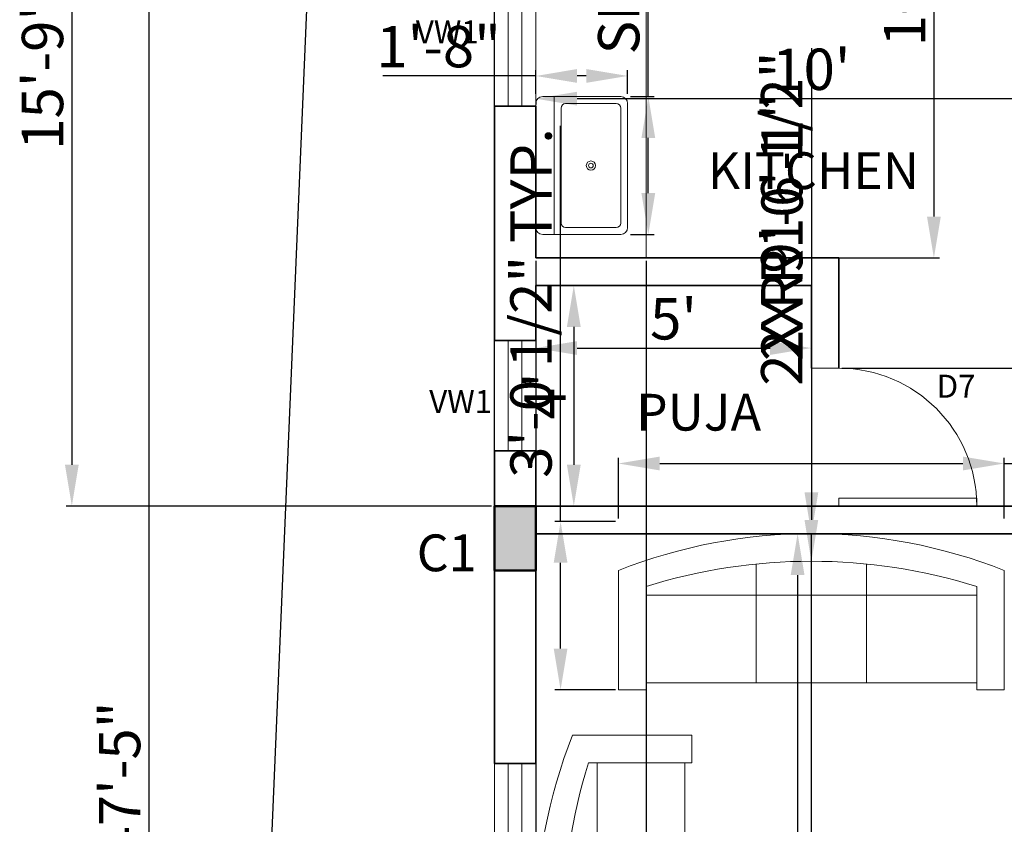
# Model space of a CAD drawing. Units: inches. Extents: x 2621 to 6190, y 513 to 1320.
# Tile 2 of 11: x 2675 to 2889, y 828 to 1003. Entities that reach past the tile are written whole.
import ezdxf

# ---------------------------------------------------------------- set-up
doc = ezdxf.new("R2010")
doc.units = ezdxf.units.IN
for name, color, linetype, lineweight in [('A-ANNO-DIMS', 5, 'Continuous', 18), ('A-ANNO-TEXT', 7, 'Continuous', 18), ('A-AREA-IDEN', 7, 'Continuous', 25), ('A-FLOR-CASE', 30, 'Continuous', 18), ('A-FLOR-FIXT', 30, 'Continuous', 18), ('A-WALL', 7, 'Continuous', 35), ('C-PROP', 7, 'Continuous', 25), ('columns', 2, 'Continuous', 50), ('door', 1, 'Continuous', 18), ('furniture', 30, 'Continuous', 18), ('S-COLS-IDEN', 2, 'Continuous', 25), ('S-COLS-PATT', 2, 'Continuous', 13), ('window', 172, 'Continuous', 18)]:
    doc.layers.add(name, color=color, linetype=linetype, lineweight=lineweight)
doc.styles.get("Standard").update_dxf_attribs({"font": 'arial.ttf'})
doc.dimstyles.new('ISO-25', dxfattribs={"dimtxt": 9, "dimasz": 9, "dimexe": 1.25, "dimexo": 0.625, "dimtad": 1, "dimlunit": 3, "dimtxsty": 'Standard', "dimcen": 2.5, "dimadec": 0, "dimazin": 0, "dimtfac": 1, "dimtmove": 0, "dimatfit": 3, "dimfxl": 1, "dimarcsym": 0})

# ---------------------------------------------------------------- blocks, each defined once
blk = doc.blocks.new('*U1')
for p, q in [((0, 0), (0, -6)), ((30, 0), (30, -6))]:
    blk.add_line(p, q)
blk.add_lwpolyline([(0, 0), (0, 30), (1.75, 30), (1.75, 0)], close=True)
blk.add_arc((0, 0), 30, 0, 90)
blk = doc.blocks.new('Sofa - Roundback 7 ft.')
for p, q in [((-12.00002, -32.4421), (-12.00003, -6.5971)), ((11.99997, -32.4421), (11.99998, -6.5971)), ((-36.000027, -34), (-36.000027, -11.4696)), ((35.99998, -34), (35.99998, -11.4696)), ((-35.999844, -13.3819), (35.9998, -13.3819)), ((-36.000027, -32.4421), (35.99998, -32.4421))]:
    blk.add_line(p, q)
for points in [[(-36.000027, -34), (-42.000027, -34), (-42.000027, -8)], [(41.99998, -8), (41.99998, -34), (35.99998, -34)]]:
    blk.add_lwpolyline(points)
for centre, radius, start, end in [((0, -114.25), 114.25, 68.43141, 111.5686), ((-0.00001, -127.1968), 121.1968, 72.72033, 107.2797)]:
    blk.add_arc(centre, radius, start, end)
blk = doc.blocks.new('Sink-single - 30 in top')
blk.add_line((-15, -3.999996), (15, -3.999996))
for points in [[(-13.5, 0), (13.5, 0)], [(-15, -18.499996), (-15, -1.5)], [(15, -1.5), (15, -18.499996)], [(-12.5, -5.499996), (12.5, -5.499996)], [(-13.5, -17.499996), (-13.5, -6.499996)], [(13.5, -6.499996), (13.5, -17.499996)], [(12.5, -18.499996), (-12.5, -18.499996)], [(13.5, -19.999996), (-13.5, -19.999996)]]:
    blk.add_lwpolyline(points)
for radius in [1, 0.5]:
    blk.add_circle((0, -11.999996), radius)
for centre, radius, start, end in [((-13.5, -1.5), 1.5, 90, 180), ((13.5, -1.5), 1.5, 0, 90), ((-12.5, -6.499996), 1, 90, 180), ((12.5, -6.499996), 1, 0, 90), ((-13.5, -18.499996), 1.5, 180, 270), ((-12.5, -17.499996), 1, 180, 270), ((12.5, -17.499996), 1, 270, 0), ((13.5, -18.499996), 1.5, 270, 0)]:
    blk.add_arc(centre, radius, start, end)
blk = doc.blocks.new('*D18')
at = {"layer": 'A-ANNO-DIMS', "color": 0, "lineweight": -2, "transparency": 16777216}
for p, q in [((2820.57, 1076.89), (2875.3, 1076.89)), ((2874.05, 1067.89), (2874.05, 959.89)), ((2820.57, 950.89), (2875.3, 950.89))]:
    blk.add_line(p, q, dxfattribs=at)
at = {"layer": 'A-ANNO-DIMS', "color": 0, "transparency": 16777216}
for points in [[(2872.55, 1067.89), (2875.55, 1067.89), (2874.05, 1076.89)], [(2872.55, 959.89), (2875.55, 959.89), (2874.05, 950.89)]]:
    blk.add_solid(points, dxfattribs=at)
at = {"layer": 'Defpoints', "color": 0, "transparency": 16777216}
for p in [(2819.94, 1076.89), (2819.94, 950.89), (2874.05, 950.89)]:
    blk.add_point(p, dxfattribs=at)
at = {"layer": 'A-ANNO-DIMS', "color": 0, "transparency": 16777216, "insert": (2868.83, 1013.89), "char_height": 9, "attachment_point": 5, "rotation": 90}
blk.add_mtext('10\'-6"', dxfattribs=at)
blk = doc.blocks.new('*D19')
at = {"layer": 'A-ANNO-DIMS', "color": 0, "lineweight": -2, "transparency": 16777216}
for p, q in [((2787.38, 984.93), (2787.38, 984.3)), ((2796.38, 985.55), (2898.38, 985.55)), ((2907.38, 984.93), (2907.38, 984.3))]:
    blk.add_line(p, q, dxfattribs=at)
at = {"layer": 'A-ANNO-DIMS', "color": 0, "transparency": 16777216}
for points in [[(2796.38, 987.05), (2796.38, 984.05), (2787.38, 985.55)], [(2898.38, 987.05), (2898.38, 984.05), (2907.38, 985.55)]]:
    blk.add_solid(points, dxfattribs=at)
at = {"layer": 'Defpoints', "color": 0, "transparency": 16777216}
for p in [(2787.38, 985.55), (2907.38, 985.55), (2907.38, 985.55)]:
    blk.add_point(p, dxfattribs=at)
at = {"layer": 'A-ANNO-DIMS', "color": 0, "transparency": 16777216, "insert": (2847.38, 990.77), "char_height": 9, "attachment_point": 5}
blk.add_mtext("10'", dxfattribs=at)
blk = doc.blocks.new('*D25')
at = {"layer": 'A-ANNO-DIMS', "color": 0, "lineweight": -2, "transparency": 16777216}
for p, q in [((2826.27, 890.89), (2845.63, 890.89)), ((2844.38, 881.89), (2844.38, 719.89)), ((2826.27, 710.89), (2845.63, 710.89))]:
    blk.add_line(p, q, dxfattribs=at)
at = {"layer": 'A-ANNO-DIMS', "color": 0, "transparency": 16777216}
for points in [[(2842.88, 881.89), (2845.88, 881.89), (2844.38, 890.89)], [(2842.88, 719.89), (2845.88, 719.89), (2844.38, 710.89)]]:
    blk.add_solid(points, dxfattribs=at)
at = {"layer": 'Defpoints', "color": 0, "transparency": 16777216}
for p in [(2825.64, 890.89), (2825.64, 710.89), (2844.38, 710.89)]:
    blk.add_point(p, dxfattribs=at)
at = {"layer": 'A-ANNO-DIMS', "color": 0, "transparency": 16777216, "insert": (2839.16, 800.89), "char_height": 9, "attachment_point": 5, "rotation": 90}
blk.add_mtext("15'", dxfattribs=at)
blk = doc.blocks.new('*D40')
at = {"layer": 'A-ANNO-DIMS', "color": 0, "lineweight": -2, "transparency": 16777216}
for p, q in [((2741.76, 1121.89), (2701.89, 1121.89)), ((2703.14, 1112.89), (2703.14, 561.89)), ((2717.76, 552.89), (2701.89, 552.89))]:
    blk.add_line(p, q, dxfattribs=at)
at = {"layer": 'A-ANNO-DIMS', "color": 0, "transparency": 16777216}
for points in [[(2701.64, 1112.89), (2704.64, 1112.89), (2703.14, 1121.89)], [(2701.64, 561.89), (2704.64, 561.89), (2703.14, 552.89)]]:
    blk.add_solid(points, dxfattribs=at)
at = {"layer": 'Defpoints', "color": 0, "transparency": 16777216}
for p in [(2742.38, 1121.89), (2703.14, 552.89), (2718.38, 552.89)]:
    blk.add_point(p, dxfattribs=at)
at = {"layer": 'A-ANNO-DIMS', "color": 0, "transparency": 16777216, "insert": (2697.94, 837.39), "char_height": 9, "attachment_point": 5, "rotation": 90}
blk.add_mtext('47\'-5"', dxfattribs=at)
blk = doc.blocks.new('*D41')
at = {"layer": 'A-ANNO-DIMS', "color": 0, "lineweight": -2, "transparency": 16777216}
for p, q in [((2788.01, 944.89), (2796.91, 944.89)), ((2795.66, 935.89), (2795.66, 905.89)), ((2788.01, 896.89), (2796.91, 896.89))]:
    blk.add_line(p, q, dxfattribs=at)
at = {"layer": 'A-ANNO-DIMS', "color": 0, "transparency": 16777216}
for points in [[(2794.16, 935.89), (2797.16, 935.89), (2795.66, 944.89)], [(2794.16, 905.89), (2797.16, 905.89), (2795.66, 896.89)]]:
    blk.add_solid(points, dxfattribs=at)
at = {"layer": 'Defpoints', "color": 0, "transparency": 16777216}
for p in [(2787.38, 944.89), (2787.38, 896.89), (2795.66, 896.89)]:
    blk.add_point(p, dxfattribs=at)
at = {"layer": 'A-ANNO-DIMS', "color": 0, "transparency": 16777216, "insert": (2790.54, 920.89), "char_height": 9, "attachment_point": 5, "rotation": 90}
blk.add_mtext("4'", dxfattribs=at)
blk = doc.blocks.new('*D42')
at = {"layer": 'A-ANNO-DIMS', "color": 0, "lineweight": -2, "transparency": 16777216}
for p, q in [((2787.38, 944.26), (2787.38, 930.03)), ((2847.38, 944.26), (2847.38, 930.03)), ((2796.38, 931.28), (2838.38, 931.28))]:
    blk.add_line(p, q, dxfattribs=at)
at = {"layer": 'A-ANNO-DIMS', "color": 0, "transparency": 16777216}
for points in [[(2796.38, 932.78), (2796.38, 929.78), (2787.38, 931.28)], [(2838.38, 932.78), (2838.38, 929.78), (2847.38, 931.28)]]:
    blk.add_solid(points, dxfattribs=at)
at = {"layer": 'Defpoints', "color": 0, "transparency": 16777216}
for p in [(2787.38, 944.89), (2847.38, 944.89), (2847.38, 931.28)]:
    blk.add_point(p, dxfattribs=at)
at = {"layer": 'A-ANNO-DIMS', "color": 0, "transparency": 16777216, "insert": (2817.38, 936.48), "char_height": 9, "attachment_point": 5}
blk.add_mtext("5'", dxfattribs=at)
blk = doc.blocks.new('WIN-VENT-24IN')
for p, q in [((9, 24), (0, 24)), ((0, 24), (0, 0)), ((3, 24), (3, 0)), ((6, 24), (6, 0)), ((9, 0), (9, 24)), ((0, 0), (9, 0))]:
    blk.add_line(p, q)
blk = doc.blocks.new('WIN-48IN')
for p, q in [((48, 9), (0, 9)), ((0, 9), (0, 0)), ((48, 0), (48, 9)), ((0, 6), (48, 6)), ((0, 3), (48, 3)), ((0, 0), (48, 0))]:
    blk.add_line(p, q)
blk = doc.blocks.new('*D65')
at = {"layer": 'A-ANNO-DIMS', "color": 0, "lineweight": -2, "transparency": 16777216}
for p, q in [((2805.38, 894.18), (2805.38, 907.41)), ((2889.38, 894.18), (2889.38, 907.41)), ((2814.38, 906.16), (2880.38, 906.16)), ((2889.38, 906.16), (2992.17, 906.16))]:
    blk.add_line(p, q, dxfattribs=at)
at = {"layer": 'A-ANNO-DIMS', "color": 0, "transparency": 16777216}
for points in [[(2814.38, 907.66), (2814.38, 904.66), (2805.38, 906.16)], [(2880.38, 907.66), (2880.38, 904.66), (2889.38, 906.16)]]:
    blk.add_solid(points, dxfattribs=at)
at = {"layer": 'Defpoints', "color": 0, "transparency": 16777216}
for p in [(2889.38, 906.16), (2805.38, 893.56), (2889.38, 893.56)]:
    blk.add_point(p, dxfattribs=at)
at = {"layer": 'A-ANNO-DIMS', "color": 0, "transparency": 16777216, "insert": (2945.28, 911.44), "char_height": 9, "attachment_point": 5}
blk.add_mtext('SOFA 7\'-0" TYP.', dxfattribs=at)
blk = doc.blocks.new('*D66')
at = {"layer": 'A-ANNO-DIMS', "color": 0, "lineweight": -2, "transparency": 16777216}
for p, q in [((2792.78, 893.56), (2792.78, 979.63)), ((2804.76, 893.56), (2791.53, 893.56)), ((2792.78, 865.89), (2792.78, 884.56)), ((2804.76, 856.89), (2791.53, 856.89))]:
    blk.add_line(p, q, dxfattribs=at)
at = {"layer": 'A-ANNO-DIMS', "color": 0, "transparency": 16777216}
for points in [[(2791.28, 884.56), (2794.28, 884.56), (2792.78, 893.56)], [(2791.28, 865.89), (2794.28, 865.89), (2792.78, 856.89)]]:
    blk.add_solid(points, dxfattribs=at)
at = {"layer": 'Defpoints', "color": 0, "transparency": 16777216}
for p in [(2792.78, 893.56), (2805.38, 893.56), (2805.38, 856.89)]:
    blk.add_point(p, dxfattribs=at)
at = {"layer": 'A-ANNO-DIMS', "color": 0, "transparency": 16777216, "insert": (2787.5, 941.09), "char_height": 9, "attachment_point": 5, "rotation": 90}
blk.add_mtext('3\'-0 1/2" TYP.', dxfattribs=at)
blk = doc.blocks.new('*D77')
at = {"layer": 'A-ANNO-DIMS', "color": 0, "lineweight": -2, "transparency": 16777216}
for p, q in [((2811.88, 985.99), (2811.88, 1052.96)), ((2808.01, 985.99), (2813.13, 985.99)), ((2811.88, 964.99), (2811.88, 976.99)), ((2808.01, 955.99), (2813.13, 955.99))]:
    blk.add_line(p, q, dxfattribs=at)
at = {"layer": 'A-ANNO-DIMS', "color": 0, "transparency": 16777216}
for points in [[(2810.38, 976.99), (2813.38, 976.99), (2811.88, 985.99)], [(2810.38, 964.99), (2813.38, 964.99), (2811.88, 955.99)]]:
    blk.add_solid(points, dxfattribs=at)
at = {"layer": 'Defpoints', "color": 0, "transparency": 16777216}
for p in [(2807.38, 985.99), (2811.88, 985.99), (2807.38, 955.99)]:
    blk.add_point(p, dxfattribs=at)
at = {"layer": 'A-ANNO-DIMS', "color": 0, "transparency": 16777216, "insert": (2806.6, 1023.98), "char_height": 9, "attachment_point": 5, "rotation": 90}
blk.add_mtext('SINK 2\'-6"', dxfattribs=at)
blk = doc.blocks.new('*D78')
at = {"layer": 'A-ANNO-DIMS', "color": 0, "lineweight": -2, "transparency": 16777216}
for p, q in [((2787.38, 990.49), (2754.05, 990.49)), ((2787.38, 986.62), (2787.38, 991.74)), ((2798.38, 990.49), (2796.38, 990.49)), ((2807.38, 986.62), (2807.38, 991.74))]:
    blk.add_line(p, q, dxfattribs=at)
at = {"layer": 'A-ANNO-DIMS', "color": 0, "transparency": 16777216}
for points in [[(2796.38, 991.99), (2796.38, 988.99), (2787.38, 990.49)], [(2798.38, 991.99), (2798.38, 988.99), (2807.38, 990.49)]]:
    blk.add_solid(points, dxfattribs=at)
at = {"layer": 'Defpoints', "color": 0, "transparency": 16777216}
for p in [(2787.38, 990.49), (2787.38, 985.99), (2807.38, 985.99)]:
    blk.add_point(p, dxfattribs=at)
at = {"layer": 'A-ANNO-DIMS', "color": 0, "transparency": 16777216, "insert": (2766.22, 995.71), "char_height": 9, "attachment_point": 5}
blk.add_mtext('1\'-8"', dxfattribs=at)
blk = doc.blocks.new('*D81')
at = {"layer": 'A-ANNO-DIMS', "color": 0, "lineweight": -2, "transparency": 16777216}
for p, q in [((2777.76, 1085.89), (2685.13, 1085.89)), ((2686.38, 1076.89), (2686.38, 905.89)), ((2777.76, 896.89), (2685.13, 896.89))]:
    blk.add_line(p, q, dxfattribs=at)
at = {"layer": 'A-ANNO-DIMS', "color": 0, "transparency": 16777216}
for points in [[(2684.88, 1076.89), (2687.88, 1076.89), (2686.38, 1085.89)], [(2684.88, 905.89), (2687.88, 905.89), (2686.38, 896.89)]]:
    blk.add_solid(points, dxfattribs=at)
at = {"layer": 'Defpoints', "color": 0, "transparency": 16777216}
for p in [(2778.38, 1085.89), (2686.38, 896.89), (2778.38, 896.89)]:
    blk.add_point(p, dxfattribs=at)
at = {"layer": 'A-ANNO-DIMS', "color": 0, "transparency": 16777216, "insert": (2681.16, 991.39), "char_height": 9, "attachment_point": 5, "rotation": 90}
blk.add_mtext('15\'-9"', dxfattribs=at)
blk = doc.blocks.new('*D87')
at = {"layer": 'A-ANNO-DIMS', "color": 0, "lineweight": -2, "transparency": 16777216}
for p, q in [((2778.38, 897.51), (2778.38, 1155.14)), ((2787.38, 1153.89), (2901.22, 1153.89)), ((2910.22, 898.87), (2910.22, 1155.14))]:
    blk.add_line(p, q, dxfattribs=at)
at = {"layer": 'A-ANNO-DIMS', "color": 0, "transparency": 16777216}
for points in [[(2787.38, 1155.39), (2787.38, 1152.39), (2778.38, 1153.89)], [(2901.22, 1155.39), (2901.22, 1152.39), (2910.22, 1153.89)]]:
    blk.add_solid(points, dxfattribs=at)
at = {"layer": 'Defpoints', "color": 0, "transparency": 16777216}
for p in [(2910.22, 1153.89), (2910.22, 898.24), (2778.38, 896.89)]:
    blk.add_point(p, dxfattribs=at)
at = {"layer": 'A-ANNO-DIMS', "color": 0, "transparency": 16777216, "insert": (2844.3, 1159.11), "char_height": 9, "attachment_point": 5}
blk.add_mtext('11\'-0"', dxfattribs=at)
blk = doc.blocks.new('*D93')
at = {"layer": 'A-ANNO-DIMS', "color": 0, "lineweight": -2, "transparency": 16777216}
for p, q in [((2787.38, 950.26), (2787.38, 519.64)), ((2811.38, 950.26), (2811.38, 519.64)), ((2796.38, 520.89), (2802.38, 520.89)), ((2811.38, 520.89), (2845.71, 520.89))]:
    blk.add_line(p, q, dxfattribs=at)
at = {"layer": 'A-ANNO-DIMS', "color": 0, "transparency": 16777216}
for points in [[(2796.38, 522.39), (2796.38, 519.39), (2787.38, 520.89)], [(2802.38, 522.39), (2802.38, 519.39), (2811.38, 520.89)]]:
    blk.add_solid(points, dxfattribs=at)
at = {"layer": 'Defpoints', "color": 0, "transparency": 16777216}
for p in [(2787.38, 950.89), (2811.38, 950.89), (2811.38, 520.89)]:
    blk.add_point(p, dxfattribs=at)
at = {"layer": 'A-ANNO-DIMS', "color": 0, "transparency": 16777216, "insert": (2833.04, 526.11), "char_height": 9, "attachment_point": 5}
blk.add_mtext('2\'-0"', dxfattribs=at)
blk = doc.blocks.new('*D100')
at = {"layer": 'A-ANNO-DIMS', "color": 0, "lineweight": -2, "transparency": 16777216}
for p, q in [((2854.01, 926.89), (3291.63, 926.89)), ((3290.38, 905.89), (3290.38, 917.89)), ((2854.01, 896.89), (3291.63, 896.89))]:
    blk.add_line(p, q, dxfattribs=at)
at = {"layer": 'A-ANNO-DIMS', "color": 0, "transparency": 16777216}
for points in [[(3288.88, 917.89), (3291.88, 917.89), (3290.38, 926.89)], [(3288.88, 905.89), (3291.88, 905.89), (3290.38, 896.89)]]:
    blk.add_solid(points, dxfattribs=at)
at = {"layer": 'Defpoints', "color": 0, "transparency": 16777216}
for p in [(2853.38, 926.89), (3290.38, 926.89), (2853.38, 896.89)]:
    blk.add_point(p, dxfattribs=at)
at = {"layer": 'A-ANNO-DIMS', "color": 0, "transparency": 16777216, "insert": (3285.16, 911.89), "char_height": 9, "attachment_point": 5, "rotation": 90}
blk.add_mtext('2\'-6"', dxfattribs=at)
blk = doc.blocks.new('*D113')
at = {"layer": 'A-ANNO-DIMS', "color": 0, "lineweight": -2, "transparency": 16777216}
for p, q in [((2847.38, 987.74), (2847.38, 893.89)), ((2847.38, 763.69), (2847.38, 884.89))]:
    blk.add_line(p, q, dxfattribs=at)
at = {"layer": 'A-ANNO-DIMS', "color": 0, "transparency": 16777216}
blk.add_solid([(2845.88, 893.89), (2848.88, 893.89), (2847.38, 884.89)], dxfattribs=at)
at = {"layer": 'Defpoints', "color": 0, "transparency": 16777216}
for p in [(2847.38, 884.89), (2847.38, 763.69)]:
    blk.add_point(p, dxfattribs=at)
at = {"layer": 'A-ANNO-DIMS', "color": 0, "transparency": 16777216, "insert": (2842.16, 957.61), "char_height": 9, "attachment_point": 5, "rotation": 90}
blk.add_mtext('2X R10\'-1"', dxfattribs=at)
blk = doc.blocks.new('*D114')
at = {"layer": 'A-ANNO-DIMS', "color": 0, "lineweight": -2, "transparency": 16777216}
for p, q in [((2847.38, 996.56), (2847.38, 899.89)), ((2847.38, 776.64), (2847.38, 890.89))]:
    blk.add_line(p, q, dxfattribs=at)
at = {"layer": 'A-ANNO-DIMS', "color": 0, "transparency": 16777216}
blk.add_solid([(2845.88, 899.89), (2848.88, 899.89), (2847.38, 890.89)], dxfattribs=at)
at = {"layer": 'Defpoints', "color": 0, "transparency": 16777216}
for p in [(2847.38, 890.89), (2847.38, 776.64)]:
    blk.add_point(p, dxfattribs=at)
at = {"layer": 'A-ANNO-DIMS', "color": 0, "transparency": 16777216, "insert": (2842.1, 959.44), "char_height": 9, "attachment_point": 5, "rotation": 90}
blk.add_mtext('2X R9\'-6 1/2"', dxfattribs=at)

msp = doc.modelspace()

# ---------------------------------------------------------------- hatches: boundary and pattern name
at = {"layer": 'S-COLS-PATT'}
h = msp.add_hatch(color=256, dxfattribs=at)
h.dxf.hatch_style = 1
h.paths.add_polyline_path([(2787.381, 1085.89), (2778.381, 1085.89), (2778.381, 1071.89), (2787.381, 1071.89)])
h.paths.add_polyline_path([(3222.381, 1085.89), (3208.381, 1085.89), (3208.381, 1076.89), (3222.381, 1076.89)])
h.paths.add_polyline_path([(3041.381, 1085.89), (3027.381, 1085.89), (3027.381, 1076.89), (3041.381, 1076.89)])
h.paths.add_polyline_path([(2916.381, 1085.89), (2907.381, 1085.89), (2907.381, 1076.89), (2916.381, 1076.89)])
h.paths.add_polyline_path([(2916.381, 1076.89), (2913.381, 1076.89), (2913.381, 1071.89), (2916.381, 1071.89)])
h.paths.add_polyline_path([(2913.381, 1076.89), (2907.381, 1076.89), (2907.381, 1071.89), (2913.381, 1071.89)])
h.paths.add_polyline_path([(2787.381, 896.89), (2778.381, 896.89), (2778.381, 882.89), (2787.381, 882.89)])
h.paths.add_polyline_path([(2924.221, 898.241), (2910.221, 898.241), (2910.221, 889.241), (2924.221, 889.241)])
h.paths.add_polyline_path([(3036.381, 896.89), (3033.381, 896.89), (3027.381, 897.385), (3027.381, 883.385), (3033.381, 883.385), (3033.381, 890.89), (3036.381, 890.89)])
h.paths.add_polyline_path([(3036.381, 890.89), (3033.381, 890.89), (3033.381, 883.385), (3036.381, 883.385)], flags=17)
h.paths.add_polyline_path([(3222.381, 897.745), (3213.381, 897.745), (3213.381, 883.745), (3222.381, 883.745)])
h.paths.add_polyline_path([(3222.381, 710.89), (3208.381, 710.89), (3208.381, 701.89), (3222.381, 701.89)])
h.paths.add_polyline_path([(3039.318, 710.89), (3021.318, 710.89), (3021.318, 701.89), (3039.318, 701.89)])
h.paths.add_polyline_path([(2796.381, 710.89), (2778.381, 710.89), (2778.381, 701.89), (2796.381, 701.89)])

# ---------------------------------------------------------------- linework, layer by layer
at = {"layer": 'A-FLOR-CASE'}
msp.add_line((2811.381, 1052.89), (2811.381, 950.89), dxfattribs=at)
at = {"layer": 'A-WALL'}
for p, q in [((2787.381, 983.89), (2778.381, 983.89)), ((2778.381, 983.89), (2778.381, 932.89)), ((2787.381, 983.89), (2787.381, 950.89)), ((2853.381, 950.89), (2787.381, 950.89)), ((2853.381, 950.89), (2853.381, 926.89)), ((2787.381, 944.89), (2787.381, 932.89)), ((2847.381, 944.89), (2787.381, 944.89)), ((2847.381, 944.89), (2847.381, 926.89)), ((2787.381, 932.89), (2778.381, 932.89)), ((2787.381, 908.89), (2778.381, 908.89)), ((2778.381, 908.89), (2778.381, 840.89)), ((2787.381, 908.89), (2787.381, 840.89)), ((2907.381, 896.89), (2787.381, 896.89)), ((2907.381, 890.89), (2787.381, 890.89)), ((2778.381, 840.89), (2787.381, 840.89))]:
    msp.add_line(p, q, dxfattribs=at)
at = {"layer": 'C-PROP'}
msp.add_lwpolyline([(3258.381, 552.89), (3258.381, 1121.89), (2742.381, 1121.89), (2718.381, 552.89)], close=True, dxfattribs=at)
at = {"layer": 'columns'}
msp.add_lwpolyline([(2778.381, 896.89), (2787.381, 896.89), (2787.381, 882.89), (2778.381, 882.89)], close=True, dxfattribs=at)

# ---------------------------------------------------------------- block references
at = {"layer": 'A-FLOR-FIXT', "rotation": 90}
msp.add_blockref('Sink-single - 30 in top', (2787.381, 970.99), dxfattribs=at)
at = {"layer": 'door', "xscale": -1, "rotation": 270}
msp.add_blockref('*U1', (2853.381, 896.89), dxfattribs=at)
at = {"layer": 'furniture'}
msp.add_blockref('Sofa - Roundback 7 ft.', (2847.381, 890.89), dxfattribs=at)
at = {"layer": 'furniture', "rotation": 90}
msp.add_blockref('Sofa - Roundback 7 ft.', (2787.381, 805.041), dxfattribs=at)
at = {"layer": 'window'}
msp.add_blockref('WIN-VENT-24IN', (2778.381, 983.89), dxfattribs=at)
for name, p, rotation in [('WIN-VENT-24IN', (2787.381, 932.89), 180), ('WIN-48IN', (2787.381, 792.89), 89.99999999999702)]:
    msp.add_blockref(name, p, dxfattribs=dict(at, rotation=rotation))

# ---------------------------------------------------------------- texts
at = {"layer": 'A-ANNO-TEXT', "char_height": 5, "attachment_point": 1}
for s, width, insert in [('VW1', 21.64382, (2761.264, 1002.569)), ('D7', 12.30066, (2874.645, 925.477)), ('VW1', 21.64382, (2764.178, 922.135))]:
    msp.add_mtext_dynamic_manual_height_columns(s, width=width, gutter_width=12.5, heights=[0], dxfattribs=dict(at, insert=insert))
at = {"layer": 'A-AREA-IDEN', "char_height": 8, "attachment_point": 1}
for s, insert in [('KITCHEN', (2824.829, 973.873)), ('PUJA', (2809.185, 921.321))]:
    msp.add_mtext_dynamic_manual_height_columns(s, width=40.12902, gutter_width=12.5, heights=[0], dxfattribs=dict(at, insert=insert))
at = {"layer": 'S-COLS-IDEN', "insert": (2761.467, 890.717), "char_height": 8, "attachment_point": 1}
msp.add_mtext_dynamic_manual_height_columns('C1', width=53.01391, gutter_width=12.5, heights=[0], dxfattribs=at)

# ---------------------------------------------------------------- dimensions: what is measured, and where the dimension line sits
at = {"layer": 'A-ANNO-DIMS'}
for base, p1, p2, override, picture, middle in [((2910.221, 1153.89), (2778.381, 896.89), (2910.221, 898.241), {"dimdec": 1, "dimlfac": 1, "dimrnd": 0, "dimzin": 1, "dimdsep": 46, "dimlunit": 4, "dimfrac": 2}, '*D87', (2844.301, 1159.11)), ((2907.381, 985.551), (2787.381, 985.551), (2907.381, 985.551), {"dimclrd": 0, "dimclre": 0, "dimclrt": 0}, '*D19', (2847.381, 990.771)), ((2811.381, 520.89), (2787.381, 950.89), (2811.381, 950.89), {"dimdec": 1, "dimlfac": 1, "dimrnd": 0, "dimzin": 1, "dimdsep": 46, "dimlunit": 4, "dimfrac": 2}, '*D93', (2833.045, 526.11))]:
    dim = msp.add_linear_dim(base=base, p1=p1, p2=p2, dimstyle='ISO-25', override=override, dxfattribs=at)
    dim.commit()
    dim.dimension.update_dxf_attribs({"geometry": picture, "text_midpoint": middle})
for base, p1, p2, angle, override, picture, middle in [((2703.139, 552.89), (2742.381, 1121.89), (2718.381, 552.89), 90, {"dimclrd": 0, "dimclre": 0, "dimclrt": 0}, '*D40', (2697.937, 837.39)), ((2686.381, 896.89), (2778.381, 1085.89), (2778.381, 896.89), 90, {"dimdec": 1, "dimlfac": 1, "dimrnd": 0, "dimzin": 1, "dimdsep": 46, "dimlunit": 4, "dimfrac": 2}, '*D81', (2681.161, 991.39)), ((2874.051, 950.89), (2819.945, 1076.89), (2819.945, 950.89), 90, {"dimclrd": 0, "dimclre": 0, "dimclrt": 0}, '*D18', (2868.831, 1013.89)), ((2787.381, 990.49), (2807.381, 985.99), (2787.381, 985.99), 180, {"dimdec": 1, "dimlfac": 1, "dimrnd": 0, "dimzin": 1, "dimdsep": 46, "dimlunit": 4, "dimfrac": 2}, '*D78', (2766.217, 995.711)), ((2795.663, 896.89), (2787.381, 944.89), (2787.381, 896.89), 90, {"dimclrd": 0, "dimclre": 0, "dimclrt": 0}, '*D41', (2790.538, 920.89)), ((3290.381, 926.89), (2853.381, 896.89), (2853.381, 926.89), 90, {"dimdec": 1, "dimlfac": 1, "dimrnd": 0, "dimzin": 1, "dimdsep": 46, "dimlunit": 4, "dimfrac": 2}, '*D100', (3285.161, 911.89)), ((2844.381, 710.89), (2825.641, 890.89), (2825.641, 710.89), 90, {"dimclrd": 0, "dimclre": 0, "dimclrt": 0}, '*D25', (2839.161, 800.89))]:
    dim = msp.add_linear_dim(base=base, p1=p1, p2=p2, angle=angle, dimstyle='ISO-25', override=override, dxfattribs=at)
    dim.commit()
    dim.dimension.update_dxf_attribs({"geometry": picture, "text_midpoint": middle})
for base, p1, p2, text, picture, middle in [((2811.881, 985.99), (2807.381, 955.99), (2807.381, 985.99), 'SINK <>', '*D77', (2806.603, 1023.975)), ((2792.781, 893.556), (2805.381, 856.89), (2805.381, 893.556), '<> TYP.', '*D66', (2787.499, 941.094))]:
    dim = msp.add_linear_dim(base=base, p1=p1, p2=p2, angle=90, text=text, dimstyle='ISO-25', override={"dimdec": 1, "dimlfac": 1, "dimrnd": 0, "dimzin": 1, "dimdsep": 46, "dimlunit": 4, "dimfrac": 2}, dxfattribs=at)
    dim.commit()
    dim.dimension.update_dxf_attribs({"geometry": picture, "text_midpoint": middle})
for center, mpoint, picture, middle in [((2847.381002, 776.639565), (2847.381, 890.889565), '*D114', (2847.381, 959.439565)), ((2847.381, 763.693), (2847.381, 884.89), '*D113', (2847.381, 957.608))]:
    dim = msp.add_radius_dim(center=center, mpoint=mpoint, text='2X <>', dimstyle='ISO-25', override={"dimdec": 1, "dimlfac": 1, "dimrnd": 0, "dimzin": 1, "dimdsep": 46, "dimlunit": 4, "dimfrac": 2}, dxfattribs=at)
    dim.commit()
    dim.dimension.update_dxf_attribs({"geometry": picture, "text_midpoint": middle, "dimtype": 164})
dim = msp.add_linear_dim(base=(2847.381, 931.282), p1=(2787.381, 944.89), p2=(2847.381, 944.89), dimstyle='ISO-25', override={"dimclrd": 0, "dimclre": 0, "dimclrt": 0}, dxfattribs=at)
dim.commit()
dim.dimension.update_dxf_attribs({"geometry": '*D42', "text_midpoint": (2817.381, 931.282), "dimtype": 160})
dim = msp.add_linear_dim(base=(2889.381, 906.156), p1=(2805.381, 893.556), p2=(2889.381, 893.556), text='SOFA <> TYP.', dimstyle='ISO-25', override={"dimdec": 1, "dimlfac": 1, "dimrnd": 0, "dimzin": 1, "dimdsep": 46, "dimlunit": 4, "dimfrac": 2}, dxfattribs=at)
dim.commit()
dim.dimension.update_dxf_attribs({"geometry": '*D65', "text_midpoint": (2945.277, 911.438)})

doc.saveas('drawing.dxf')
